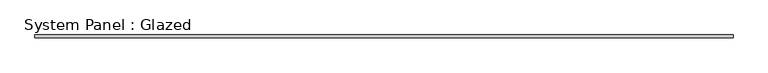
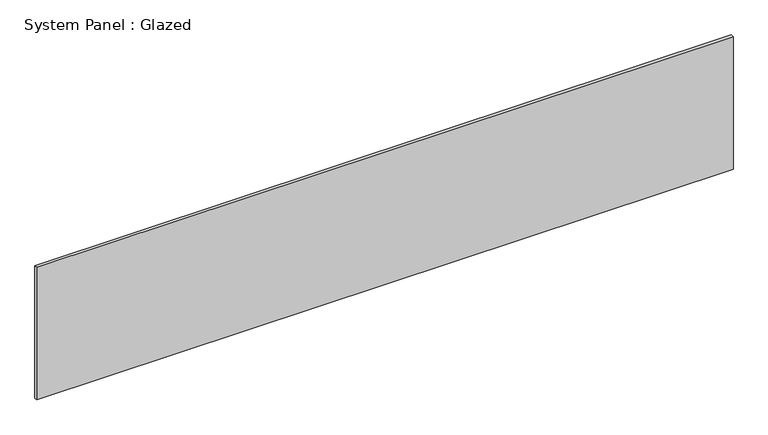
"""IFC4 building model written with IfcOpenShell, lengths in millimetres: plate geometry, System Panel : Glazed."""

from ifc_helpers import new_model, si_unit, origin, origin_with_axes, place, context, project, spatial, polyline, outline, extrude, source, transform, mapped, element, save


def system_panel_glazed_ce931456(model_context):
    return source(origin(), model_context, "Body", "SweptSolid", [
        extrude(outline(polyline([(3025.775, 19.05), (-3025.775, 19.05), (-3025.775, 44.45), (3025.775, 44.45), (3025.775, 19.05)])), origin_with_axes(), (0.0, 0.0, 1.0), 1219.2),
    ])


if __name__ == "__main__":
    model = new_model("IFC4")
    model_context = context("Model", 3, world=origin())
    ifc_project = project(units=[si_unit("LENGTHUNIT", "METRE", prefix="MILLI")], contexts=[model_context])
    site = spatial("IfcSite", under=ifc_project)
    building = spatial("IfcBuilding", under=site)
    placement = place(None, origin())
    system_panel_glazed_shape = system_panel_glazed_ce931456(model_context)
    element("IfcPlate", 1, ObjectType="System Panel : Glazed", at=placement, inside=building, context=model_context, shape_type="MappedRepresentation", body=[
        mapped(system_panel_glazed_shape, transform((0.0, 0.0, 0.0), x_axis=(1.0, 0.0, 0.0), y_axis=(0.0, 1.0, 0.0), z_axis=(0.0, 0.0, 1.0))),
    ])
    save(model, "model.ifc")

# Revit data of these elements
# Type "System Panel : Glazed"
#   Construction Type Id = "GSP4R"
#   Analytic Construction = "1/8 in Pilkington single glazing"
#   Visual Light Transmittance = 0.9
#   Solar Heat Gain Coefficient = 0.86
#   Heat Transfer Coefficient (U) = 1.18115 BTU/(h·ft²·°F)
# Element 1 (IfcPlate, "System Panel : Glazed")
#   Materials on its faces: "Glass"
# Materials
#   "Glass": class "Glass", colour RGB 0 128 192, transparency 0.75, Description = "Soda Lime Glass", Cost = 0
